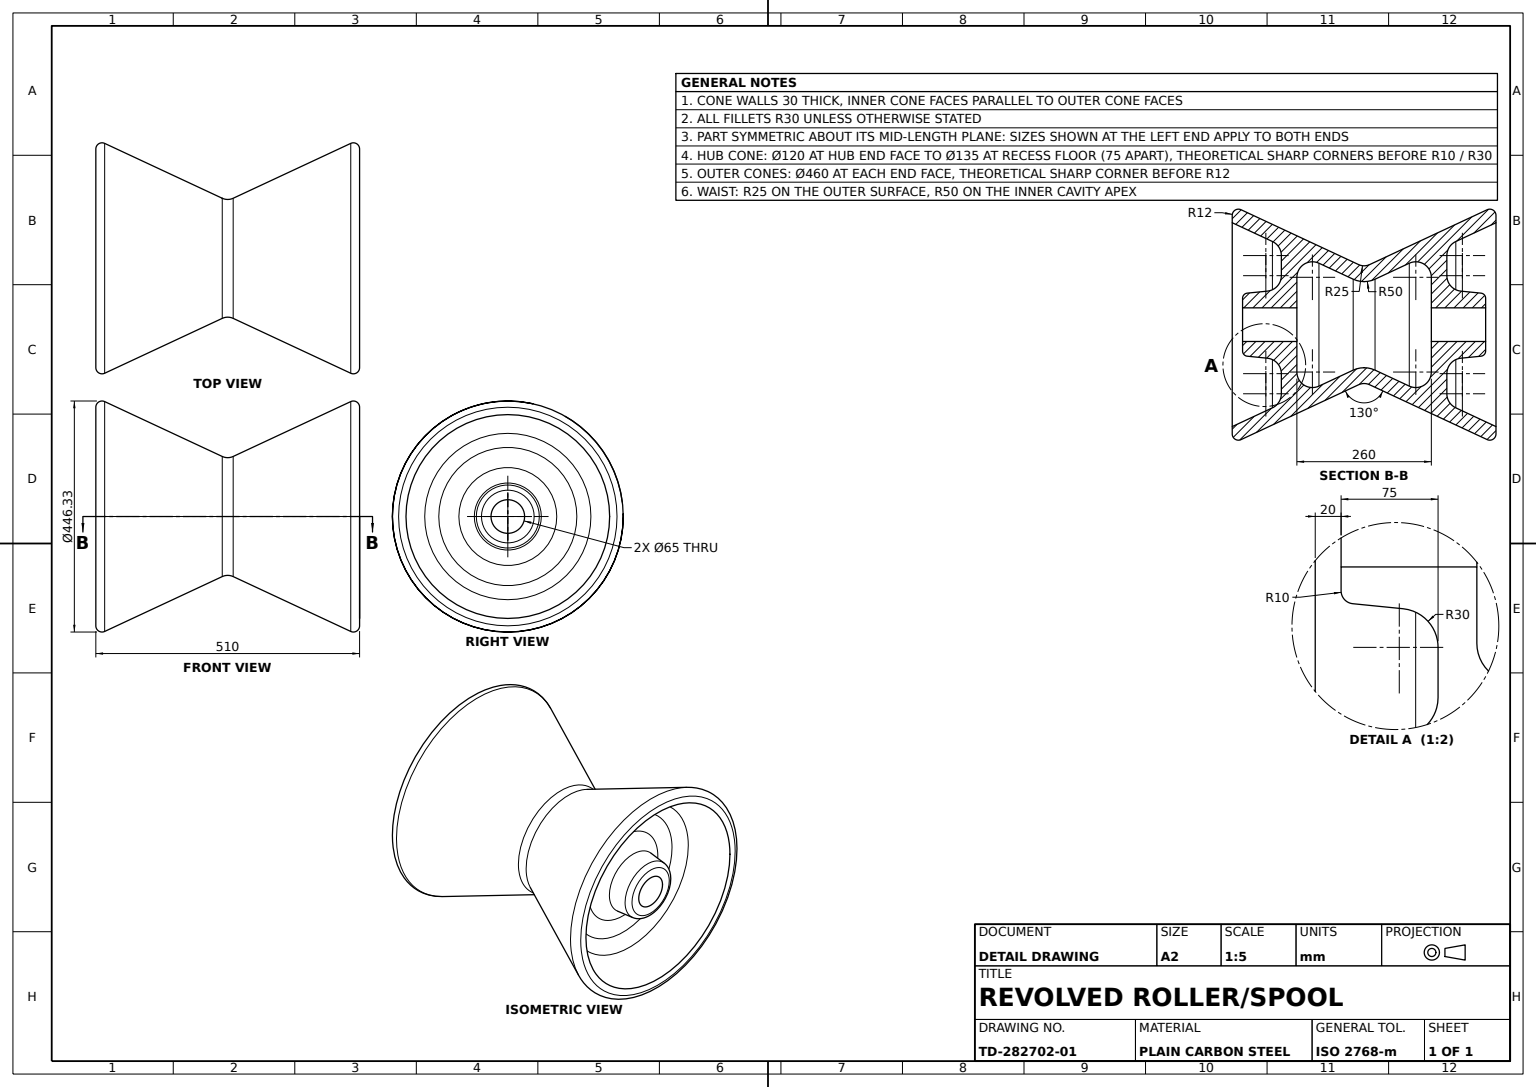
SolidWorks part; units mm, degrees
material "Plain Carbon Steel"
ref_plane "Front Plane" through (0, 0, 0) normal (0, 0, 1) x (1, 0, 0)
ref_plane "Top Plane" through (0, 0, 0) normal (0, 1, 0) x (1, 0, 0)
ref_plane "Right Plane" through (0, 0, 0) normal (1, 0, 0) x (0, 0, -1)
sketch "Pulley Profile Sketch" plane through (0, 0, 0) normal (0, 0, 1) x (1, 0, 0)
  line L0 (0, -1222.1831) -> (0, -111.0915) construction
  line L1 (0, 0) -> (101701.8425, 0) construction
  line L2 (130, 32.5) -> (235, 32.5)
  line L3 (235, 32.5) -> (235, 50.9501)
  line L6 (177.3215, 160.6766) -> (255, 196.8987)
  line L7 (255, 196.8987) -> (255, 211.1638)
  line L8 (237.9286, 222.0395) -> (10.5655, 116.0183)
  line L10 (21.1309, 87.8437) -> (87.3215, 118.7089)
  line L11 (130, 91.5196) -> (130, 32.5)
  line L12 (130, -138.6102) -> (130, -32.5) construction
  line L13 (21.1309, -87.8437) -> (130, -138.6102) construction
  line L15 (255, -230) -> (10.5655, -116.0183) construction
  line L16 (255, -196.8987) -> (255, -230) construction
  line L17 (160, -152.5994) -> (255, -196.8987) construction
  line L20 (235, -32.5) -> (235, -60) construction
  line L21 (130, -32.5) -> (235, -32.5) construction
  line L22 (225.995, 60.9005) -> (187.0149, 64.7985)
  line L23 (160, 94.6496) -> (160, 133.4873)
  line L24 (235, -60) -> (160, -67.5) construction
  line L25 (160, -67.5) -> (160, -152.5994) construction
  line L26 (-160, -67.5) -> (-160, -152.5994) construction
  line L27 (-235, -60) -> (-160, -67.5) construction
  line L28 (-160, 94.6496) -> (-160, 133.4873)
  line L29 (-225.995, 60.9005) -> (-187.0149, 64.7985)
  line L30 (-130, -32.5) -> (-235, -32.5) construction
  line L31 (-235, -32.5) -> (-235, -60) construction
  line L32 (-160, -152.5994) -> (-255, -196.8987) construction
  line L33 (-255, -196.8987) -> (-255, -230) construction
  line L34 (-255, -230) -> (-10.5655, -116.0183) construction
  line L35 (-21.1309, -87.8437) -> (-130, -138.6102) construction
  line L36 (-130, -138.6102) -> (-130, -32.5) construction
  line L37 (-130, 91.5196) -> (-130, 32.5)
  line L38 (-21.1309, 87.8437) -> (-87.3215, 118.7089)
  line L39 (-237.9286, 222.0395) -> (-10.5655, 116.0183)
  line L40 (-255, 196.8987) -> (-255, 211.1638)
  line L41 (-177.3215, 160.6766) -> (-255, 196.8987)
  line L42 (-235, 32.5) -> (-235, 50.9501)
  line L43 (-130, 32.5) -> (-235, 32.5)
  line L44 (0, 111.0915) -> (0, 101701.8425) construction
  line L45 (0, -77.9902) -> (0, 77.9902) construction
  arc A0 (-10.5655, -116.0183) -> (10.5655, -116.0183) centre (0, -138.676) cw construction
  arc A1 (21.1309, -87.8437) -> (-21.1309, -87.8437) centre (0, -133.1591) ccw construction
  arc A2 (-21.1309, 87.8437) -> (21.1309, 87.8437) centre (0, 133.1591) ccw
  arc A3 (10.5655, 116.0183) -> (-10.5655, 116.0183) centre (0, 138.676) cw
  arc A4 (-130, 91.5196) -> (-87.3215, 118.7089) centre (-100, 91.5196) cw
  arc A5 (130, 91.5196) -> (87.3215, 118.7089) centre (100, 91.5196) ccw
  arc A6 (-160, 133.4873) -> (-177.3215, 160.6766) centre (-190, 133.4873) ccw
  arc A7 (160, 133.4873) -> (177.3215, 160.6766) centre (190, 133.4873) cw
  arc A8 (-160, 94.6496) -> (-187.0149, 64.7985) centre (-190, 94.6496) cw
  arc A9 (187.0149, 64.7985) -> (160, 94.6496) centre (190, 94.6496) cw
  arc A10 (-237.9286, 222.0395) -> (-255, 211.1638) centre (-243, 211.1638) ccw
  arc A11 (255, 211.1638) -> (237.9286, 222.0395) centre (243, 211.1638) ccw
  arc A12 (-225.995, 60.9005) -> (-235, 50.9501) centre (-225, 50.9501) ccw
  arc A13 (235, 50.9501) -> (225.995, 60.9005) centre (225, 50.9501) ccw
  point P42 (255, -213.4493)
  point P58 (-130, 138.6102)
  point P61 (130, 138.6102)
  point P64 (-160, 152.5994)
  point P67 (160, 152.5994)
  point P70 (-160, 67.5)
  point P73 (160, 67.5)
  point P76 (-255, 230)
  point P79 (255, 230)
  point P82 (-235, 60)
  point P85 (235, 60)
  dimension "D10" = 25
  dimension "D11" = 50
  dimension "D12" = 50
  dimension "D13" = 25
  dimension "D15" = 30
  dimension "D16" = 30
  dimension "D17" = 30
  dimension "D18" = 12
  dimension "D19" = 10
  dimension "D1" = 65
  dimension "D2" = 120
  dimension "D3" = 135
  dimension "D4" = 460
  dimension "D5" = 30
  dimension "D6" = 75
  dimension "D7" = 260
  dimension "D8" = 510
  dimension "D9" = 130
  dimension "D14" = 30
revolve "Pulley Body Revolve" add sketch "Pulley Profile Sketch" angle 360 about L1
